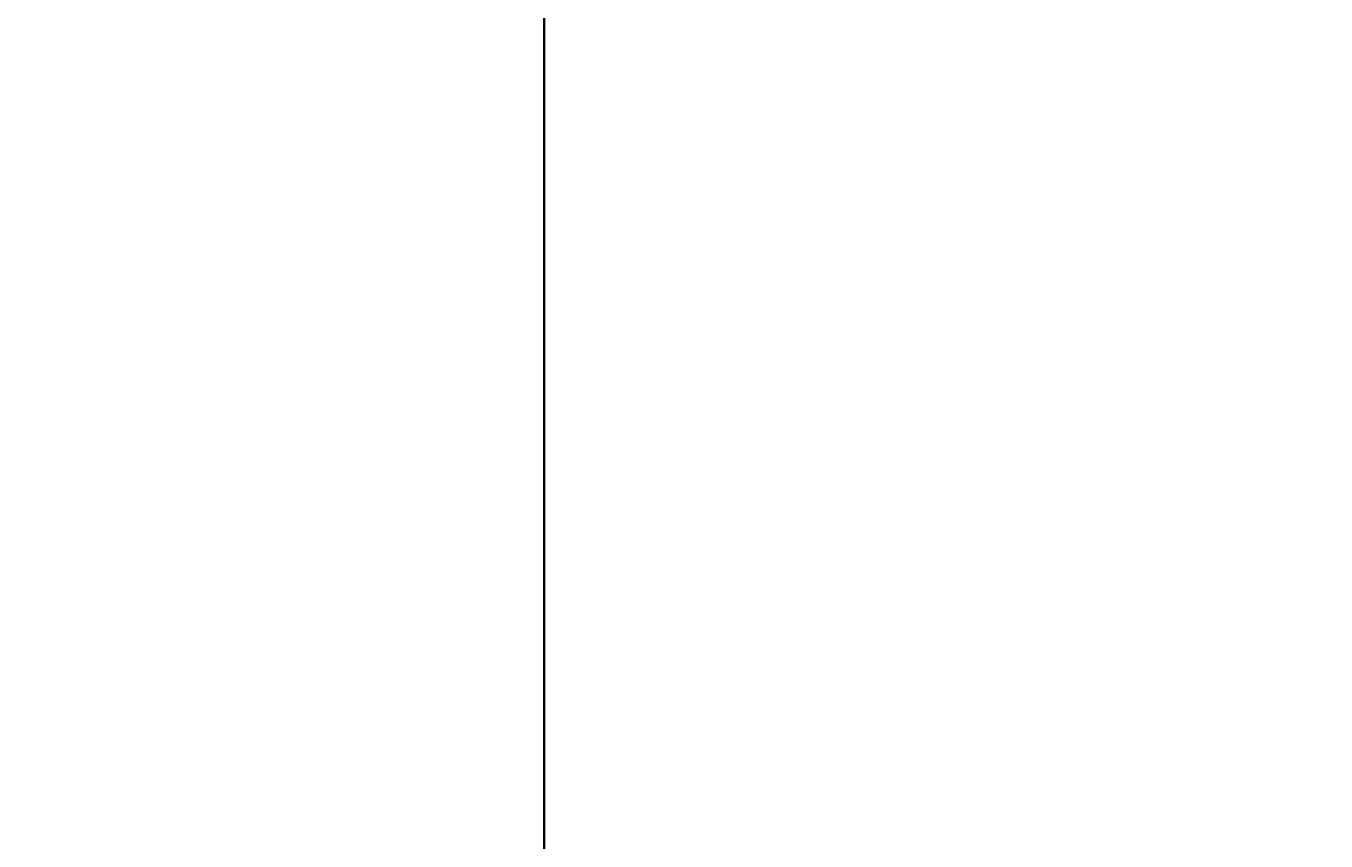
# Model space of a CAD drawing. Units: inches. Extents: x 1998 to 2588, y 1139 to 1977.
# Tile 101 of 134: x 2397 to 2425, y 1555 to 1573. Entities that reach past the tile are written whole.
import ezdxf

# ---------------------------------------------------------------- set-up
doc = ezdxf.new("R2010")
doc.units = ezdxf.units.IN
for name, color, linetype, lineweight in [('A-ANNO-DIMS', 2, 'Continuous', 18), ('A-FLOR-EVTR', 7, 'Continuous', 35), ('A-FLOR-STRS', 7, 'Continuous', 25)]:
    doc.layers.add(name, color=color, linetype=linetype, lineweight=lineweight)
doc.styles.get("Standard").update_dxf_attribs({"font": 'arial.ttf'})
doc.dimstyles.get("Standard").update_dxf_attribs({"dimtxt": 0.18, "dimasz": 0.18, "dimexe": 0.18, "dimexo": 0.0625, "dimgap": 0.09, "dimtad": 0, "dimtih": 1, "dimtoh": 1, "dimdec": 4, "dimzin": 0, "dimdsep": 46, "dimtxsty": 'Standard', "dimcen": 0.09, "dimadec": 0, "dimazin": 0, "dimtfac": 1, "dimtdec": 4, "dimtofl": 0, "dimtmove": 0, "dimatfit": 3, "dimfxl": 1, "dimtolj": 1, "dimtzin": 0, "dimarcsym": 0})

# ---------------------------------------------------------------- blocks, each defined once
blk = doc.blocks.new('*D24')
at = {"layer": 'A-ANNO-DIMS', "color": 0, "lineweight": -2, "transparency": 16777216}
for p, q in [((2398.535, 1911.232), (2588.309, 1911.232)), ((2588.129, 1911.052), (2588.129, 1570.164)), ((2588.129, 1228.912), (2588.129, 1569.8)), ((2527.535, 1228.732), (2588.309, 1228.732))]:
    blk.add_line(p, q, dxfattribs=at)
at = {"layer": 'A-ANNO-DIMS', "color": 0, "transparency": 16777216}
for points in [[(2588.099, 1911.052), (2588.159, 1911.052), (2588.129, 1911.232)], [(2588.099, 1228.912), (2588.159, 1228.912), (2588.129, 1228.732)]]:
    blk.add_solid(points, dxfattribs=at)
at = {"layer": 'Defpoints', "color": 0, "transparency": 16777216}
for p in [(2398.473, 1911.232), (2588.129, 1911.232), (2527.473, 1228.732)]:
    blk.add_point(p, dxfattribs=at)
at = {"layer": 'A-ANNO-DIMS', "color": 0, "transparency": 16777216, "insert": (2588.129, 1569.982), "char_height": 0.18, "attachment_point": 5}
blk.add_mtext('\\A1;682.5', dxfattribs=at)
blk = doc.blocks.new('*D34')
at = {"layer": 'A-ANNO-DIMS', "color": 0, "lineweight": -2, "transparency": 16777216}
for p, q in [((2407.91, 1594.732), (1997.843, 1594.732)), ((1998.023, 1594.552), (1998.023, 1558.913)), ((1998.023, 1522.912), (1998.023, 1558.552)), ((2407.91, 1522.732), (1997.843, 1522.732))]:
    blk.add_line(p, q, dxfattribs=at)
at = {"layer": 'A-ANNO-DIMS', "color": 0, "transparency": 16777216}
for points in [[(1997.993, 1594.552), (1998.053, 1594.552), (1998.023, 1594.732)], [(1997.993, 1522.912), (1998.053, 1522.912), (1998.023, 1522.732)]]:
    blk.add_solid(points, dxfattribs=at)
at = {"layer": 'Defpoints', "color": 0, "transparency": 16777216}
for p in [(1998.023, 1594.732), (2407.973, 1594.732), (2407.973, 1522.732)]:
    blk.add_point(p, dxfattribs=at)
at = {"layer": 'A-ANNO-DIMS', "color": 0, "transparency": 16777216, "insert": (1998.023, 1558.732), "char_height": 0.18, "attachment_point": 5}
blk.add_mtext('\\A1;72', dxfattribs=at)
blk = doc.blocks.new('*D42')
at = {"layer": 'A-ANNO-DIMS', "color": 0, "lineweight": -2, "transparency": 16777216}
for p, q in [((2287.535, 1588.732), (2588.309, 1588.732)), ((2588.129, 1588.552), (2588.129, 1555.914)), ((2588.129, 1522.912), (2588.129, 1555.55)), ((2287.535, 1522.732), (2588.309, 1522.732))]:
    blk.add_line(p, q, dxfattribs=at)
at = {"layer": 'A-ANNO-DIMS', "color": 0, "transparency": 16777216}
for points in [[(2588.099, 1588.552), (2588.159, 1588.552), (2588.129, 1588.732)], [(2588.099, 1522.912), (2588.159, 1522.912), (2588.129, 1522.732)]]:
    blk.add_solid(points, dxfattribs=at)
at = {"layer": 'Defpoints', "color": 0, "transparency": 16777216}
for p in [(2287.473, 1588.732), (2588.129, 1588.732), (2287.473, 1522.732)]:
    blk.add_point(p, dxfattribs=at)
at = {"layer": 'A-ANNO-DIMS', "color": 0, "transparency": 16777216, "insert": (2588.129, 1555.732), "char_height": 0.18, "attachment_point": 5}
blk.add_mtext('\\A1;66', dxfattribs=at)
blk = doc.blocks.new('*D43')
at = {"layer": 'A-ANNO-DIMS', "color": 0, "lineweight": -2, "transparency": 16777216}
for p, q in [((2407.973, 1594.67), (2407.973, 1138.602)), ((2345.973, 1588.67), (2345.973, 1138.602)), ((2346.153, 1138.782), (2376.754, 1138.782)), ((2407.793, 1138.782), (2377.191, 1138.782))]:
    blk.add_line(p, q, dxfattribs=at)
at = {"layer": 'A-ANNO-DIMS', "color": 0, "transparency": 16777216}
for points in [[(2346.153, 1138.812), (2346.153, 1138.752), (2345.973, 1138.782)], [(2407.793, 1138.812), (2407.793, 1138.752), (2407.973, 1138.782)]]:
    blk.add_solid(points, dxfattribs=at)
at = {"layer": 'Defpoints', "color": 0, "transparency": 16777216}
for p in [(2407.973, 1594.732), (2345.973, 1588.732), (2407.973, 1138.782)]:
    blk.add_point(p, dxfattribs=at)
at = {"layer": 'A-ANNO-DIMS', "color": 0, "transparency": 16777216, "insert": (2376.973, 1138.782), "char_height": 0.18, "attachment_point": 5}
blk.add_mtext('\\A1;62', dxfattribs=at)

msp = doc.modelspace()

# ---------------------------------------------------------------- linework, layer by layer
at = {"layer": 'A-FLOR-EVTR'}
msp.add_lwpolyline([(2407.9729, 1522.7324), (2498.1786, 1522.7324), (2498.1786, 1594.7324), (2407.9729, 1594.7324)], close=True, dxfattribs=at)
at = {"layer": 'A-FLOR-STRS'}
msp.add_line((2407.9729, 1480.7324), (2407.9729, 1636.7324), dxfattribs=at)

# ---------------------------------------------------------------- dimensions: what is measured, and where the dimension line sits
at = {"layer": 'A-ANNO-DIMS'}
for base, p1, p2, override, picture, middle in [((2588.1286, 1911.2324), (2527.4729, 1228.7324), (2398.4729, 1911.2324), {"dimdec": 1, "dimlfac": 1, "dimrnd": 0, "dimzin": 0, "dimdsep": 46, "dimlunit": 2}, '*D24', (2588.1286, 1569.9824)), ((1998.0229, 1594.7324), (2407.9729, 1522.7324), (2407.9729, 1594.7324), {"dimdec": 0, "dimlfac": 1, "dimrnd": 0, "dimzin": 0, "dimdsep": 46, "dimlunit": 2}, '*D34', (1998.0229, 1558.7324)), ((2588.1286, 1588.7324), (2287.4729, 1522.7324), (2287.4729, 1588.7324), {"dimdec": 0, "dimlfac": 1, "dimrnd": 0, "dimzin": 0, "dimdsep": 46, "dimlunit": 2}, '*D42', (2588.1286, 1555.7324))]:
    dim = msp.add_linear_dim(base=base, p1=p1, p2=p2, angle=90, dimstyle='Standard', override=override, dxfattribs=at)
    dim.commit()
    dim.dimension.update_dxf_attribs({"geometry": picture, "text_midpoint": middle})
dim = msp.add_linear_dim(base=(2407.9729, 1138.7824), p1=(2345.9729, 1588.7324), p2=(2407.9729, 1594.7324), dimstyle='Standard', override={"dimdec": 0, "dimlfac": 1, "dimrnd": 0, "dimzin": 0, "dimdsep": 46, "dimlunit": 2}, dxfattribs=at)
dim.commit()
dim.dimension.update_dxf_attribs({"geometry": '*D43', "text_midpoint": (2376.9729, 1138.7824)})

doc.saveas('drawing.dxf')
